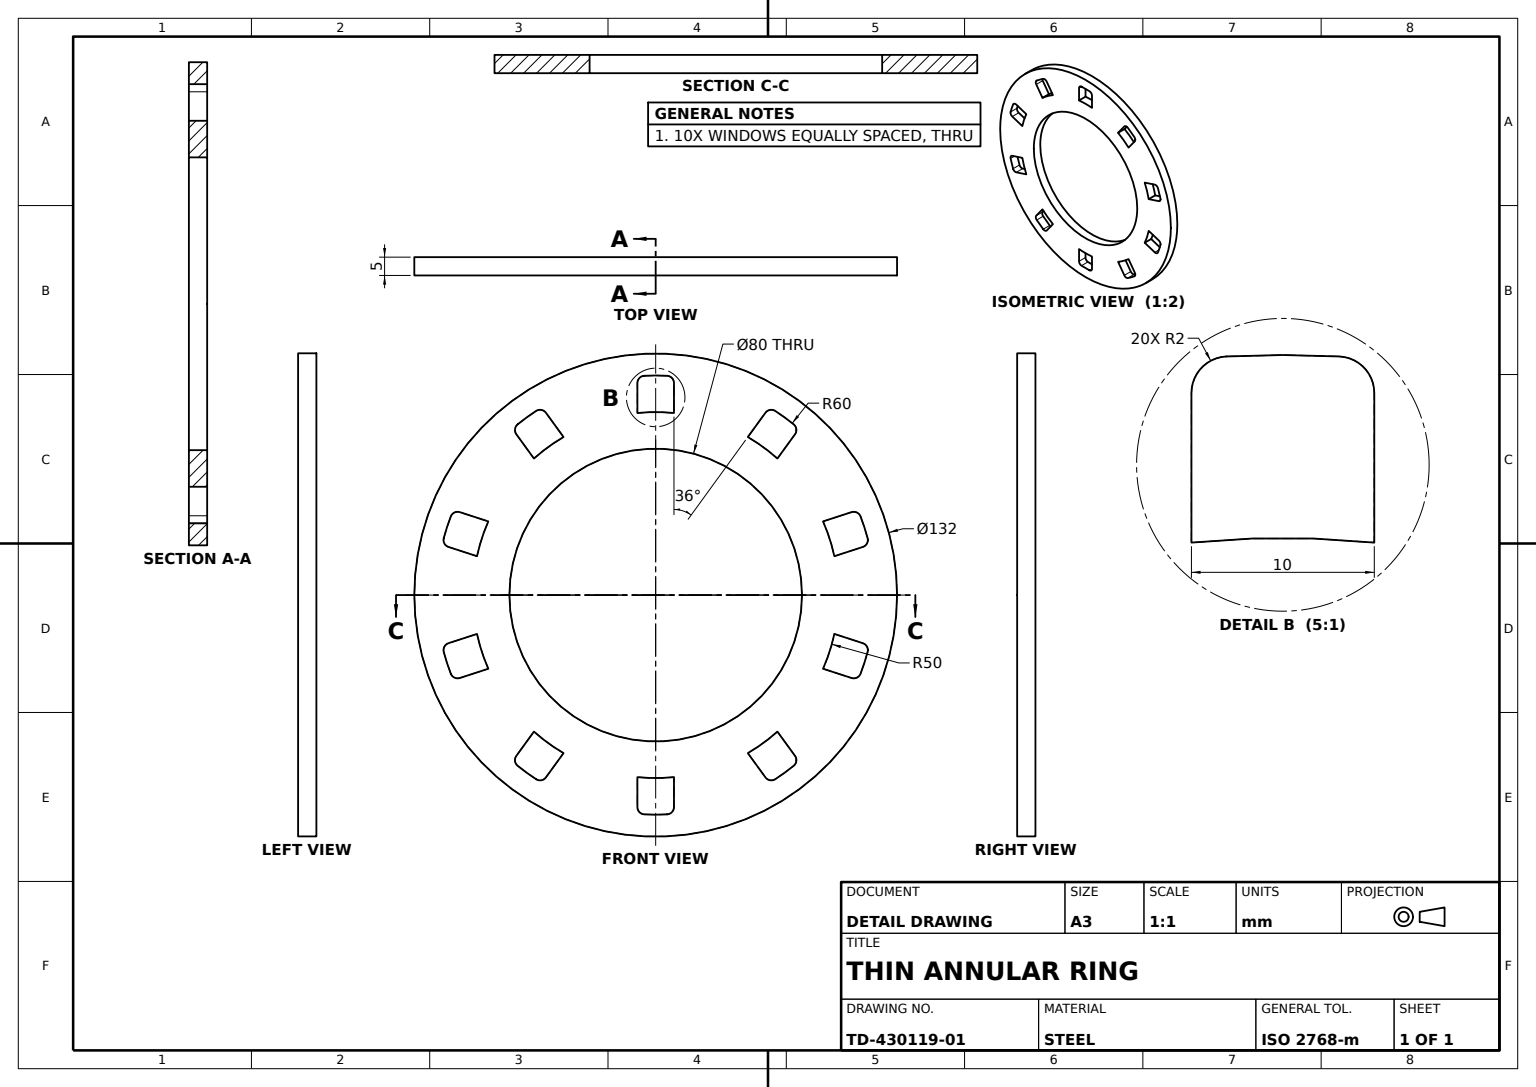
SolidWorks part; units mm, degrees
material "Plain Carbon Steel"
ref_plane "Front Plane" through (0, 0, 0) normal (0, 0, 1) x (1, 0, 0)
ref_plane "Top Plane" through (0, 0, 0) normal (0, 1, 0) x (1, 0, 0)
ref_plane "Right Plane" through (0, 0, 0) normal (1, 0, 0) x (0, 0, -1)
sketch "Ring Outline Sketch Ø132" plane through (0, 0, 0) normal (0, 0, 1) x (1, 0, 0)
  circle A0 centre (0, 0) radius 66
  dimension "D1" = 132
extrude "Ring Disc Ø132x5" add sketch "Ring Outline Sketch Ø132" along normal blind 5
sketch "Window Sketch" plane through (0, 0, 5) normal (0, 0, 1) x (1, 0, 0)
  line L1 (5, 49.7494) -> (5, 57.9224)
  line L3 (-5, 57.9224) -> (-5, 49.7494)
  arc A0 (5, 49.7494) -> (-5, 49.7494) centre (0, 0) ccw
  arc A1 (3.1034, 59.9197) -> (-3.1034, 59.9197) centre (0, 0) ccw
  arc A2 (-5, 57.9224) -> (-3.1034, 59.9197) centre (-3, 57.9224) cw
  arc A3 (5, 57.9224) -> (3.1034, 59.9197) centre (3, 57.9224) ccw
  dimension "D1" = 2
  dimension "D2" = 50
  dimension "D3" = 60
  dimension "D4" = 3
  dimension "D5" = 6
extrude "Window Cut" cut sketch "Window Sketch" against normal blind 25
pattern_circular "Window Pattern 10x" count 10 over 360 about axis through (0, 0, 0) along (0, 0, 1) of "Window Cut"
sketch "Bore Sketch Ø80" plane through (0, 0, 5) normal (0, 0, 1) x (1, 0, 0)
  circle A0 centre (0, 0) radius 40
  dimension "D1" = 80
extrude "Centre Bore Ø80" cut sketch "Bore Sketch Ø80" against normal blind 25
